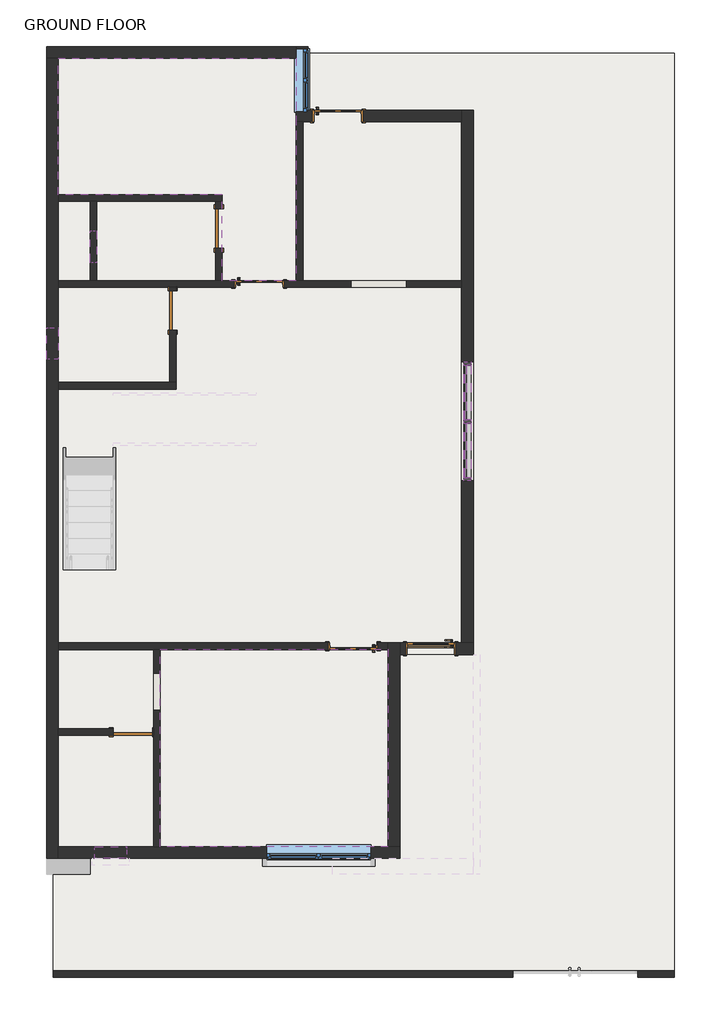
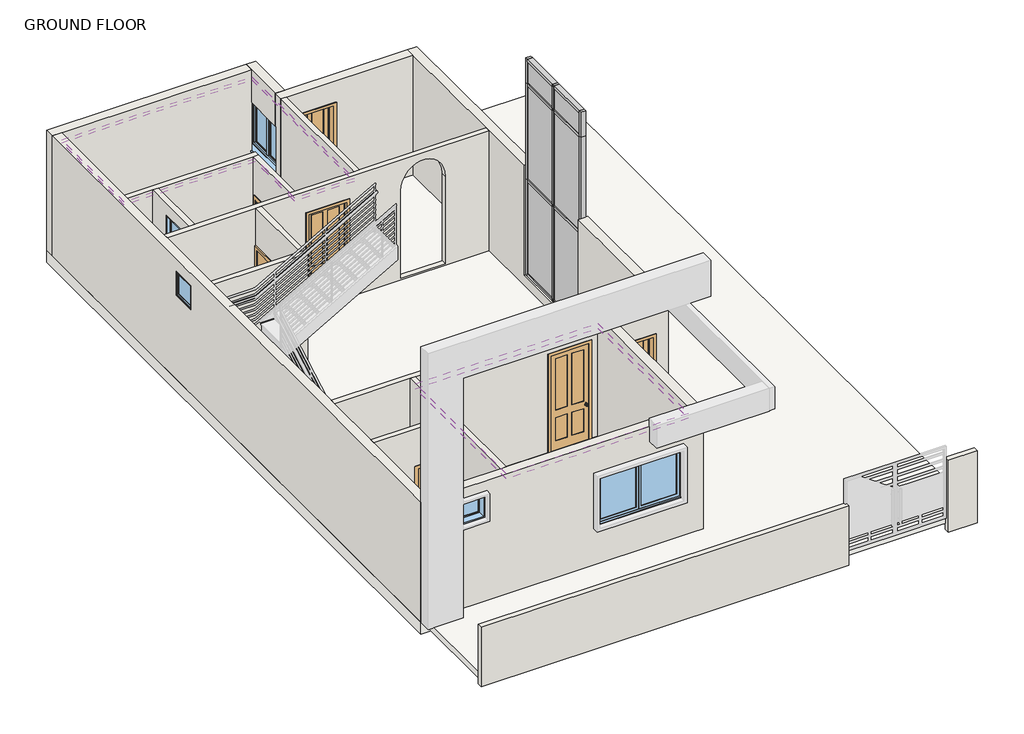
# One storey, part 1 of 3: 20 walls, 17 members, 7 doors, 6 plates, 5 windows, 4 coverings, 3 slabs.
# Revit data of these elements (continued)
# Elements 50, 51, 52, 53, 54, 55, 56, 57 (IfcWall, "OUTER WALL 9\"") (continued)
#   Base Offset = 0' - 0"
#   wall height = 10' - 0"
#   Phase Created = New Construction
#   Base Constraint = GROUND FLOOR
#   Top Constraint = FIRST FLOOR
#   Materials on its faces: "IVORY WHITE COLOUR"
# Element 58 (IfcWindow, "Fixed : 24\" x 24\"")
#   Mark = "3"
#   Phase Created = New Construction
#   Materials on its faces: "Sash", "Glass"
# Element 59 (IfcWindow, "Fixed : 24\" x 24\"")
#   Mark = "5"
#   Phase Created = New Construction
#   Materials on its faces: "Sash", "Glass"
# Element 60 (IfcWindow, "Fixed : 24\" x 24\"")
#   Mark = "4"
#   Phase Created = New Construction
#   Materials on its faces: "Sash", "Glass"
# Element 61 (IfcWindow, "w2 : window 4' x 4'")
#   Mark = "2"
#   Einbautiefe (von außen) = 0' - 5.51181"
#   Kippflügel = yes
#   Drehflügel im Grundriß darstellen = no
#   Drehflügel = yes
#   Rahmen = none
#   Glas = blue glass
#   Flügel = WINDOW COLOUR WHITE
#   Fensterbank innen = WINDOW COLOUR WHITE
#   Fensterbank aussen = WINDOW COLOUR WHITE
#   Phase Created = New Construction
#   Materials on its faces: "WINDOW COLOUR WHITE", "blue glass"
# Element 62 (IfcWindow, "w2 : window 6' x 4'")
#   Mark = "1"
#   Einbautiefe (von außen) = 0' - 5.51181"
#   Kippflügel = yes
#   Drehflügel im Grundriß darstellen = no
#   Drehflügel = yes
#   Rahmen = none
#   Glas = blue glass
#   Flügel = WINDOW COLOUR WHITE
#   Fensterbank innen = WINDOW COLOUR WHITE
#   Fensterbank aussen = WINDOW COLOUR WHITE
#   Phase Created = New Construction
#   Materials on its faces: "WINDOW COLOUR WHITE", "blue glass"
# Materials
#   "Metal Stud Layer": class "Metal", colour RGB 199 199 199, transparency 0, Description = "Light gauge steel framing, thermal air layer", Cost = 0
#   "Laminate, Ivory, Matte": class "Plastic", colour RGB 247 247 239, transparency 0, Description = "Plastic Laminate - Ivory, Matte", Cost = 0
#   "Cherry": class "Wood", colour RGB 226 177 128, transparency 0, Description = "Prunus Serotina", Cost = 0
#   "Glass": class "Glass", colour RGB 0 128 192, transparency 0.75, Description = "Soda Lime Glass", Cost = 0
#   "Aluminum": class "Metal", colour RGB 247 247 247, transparency 0, Description = "Aluminum 6061", Cost = 0
#   "Door - Panel": class "Wood", colour RGB 210 159 95, transparency 0, Cost = 0
#   "Door - Frame": colour RGB 118 70 51, transparency 0, Cost = 0
#   "VERANDA FLOORING 6\"": class "Generic", colour RGB 120 120 120, transparency 0, Cost = 0
#   "MARBLE FLOORING": class "Generic", colour RGB 120 120 120, transparency 0, Cost = 0
#   "IVORY WHITE COLOUR": class "Generic", colour RGB 120 120 120, transparency 0, Cost = 0
#   "Sash": class "Wood", colour RGB 224 178 126, transparency 0, Cost = 0
#   "blue glass": class "System", colour RGB 0 0 255, transparency 0.75, Cost = 0
#   "WINDOW COLOUR WHITE": class "Generic", colour RGB 120 120 120, transparency 0, Cost = 0
# Room at (-6191.273, -2502.487) mm, phase "New Construction", upper level "GROUND FLOOR", upper offset 10' - 0", lower offset 0' - 0"
#   Number = "1"
#   Name = "TOILET"
# Room at (-6191.273, -521.287) mm, phase "New Construction", upper level "GROUND FLOOR", upper offset 10' - 0", lower offset 0' - 0"
#   Number = "2"
# Room at (-2908.323, -1676.987) mm, phase "New Construction", upper level "GROUND FLOOR", upper offset 10' - 0", lower offset 0' - 0"
#   Number = "3"
#   Name = "BED ROOM 1"
# Room at (-831.873, 8876.713) mm, phase "New Construction", upper level "GROUND FLOOR", upper offset 10' - 0", lower offset 0' - 0"
#   Number = "4"
#   Name = "KITCHEN"
# Room at (-6038.873, 6285.913) mm, phase "New Construction", upper level "GROUND FLOOR", upper offset 10' - 0", lower offset 0' - 0"
#   Number = "5"
#   Name = "TOILET"
# Room at (-3206.773, 3758.613) mm, phase "New Construction", upper level "GROUND FLOOR", upper offset 10' - 0", lower offset 0' - 0"
#   Number = "6"
#   Name = "LIVING AND DINING HALL"
# Room at (-4794.273, 9486.313) mm, phase "New Construction", upper level "GROUND FLOOR", upper offset 10' - 0", lower offset 0' - 0"
#   Number = "7"
#   Name = "BED ROOM"
# Room at (-5200.673, 8089.313) mm, phase "New Construction", upper level "GROUND FLOOR", upper offset 10' - 0", lower offset 0' - 0"
#   Number = "8"
#   Name = "TOILET"
# Room at (-6800.873, 8089.313) mm, phase "New Construction", upper level "GROUND FLOOR", upper offset 10' - 0", lower offset 0' - 0"
#   Number = "9"
#   Name = "Room"
